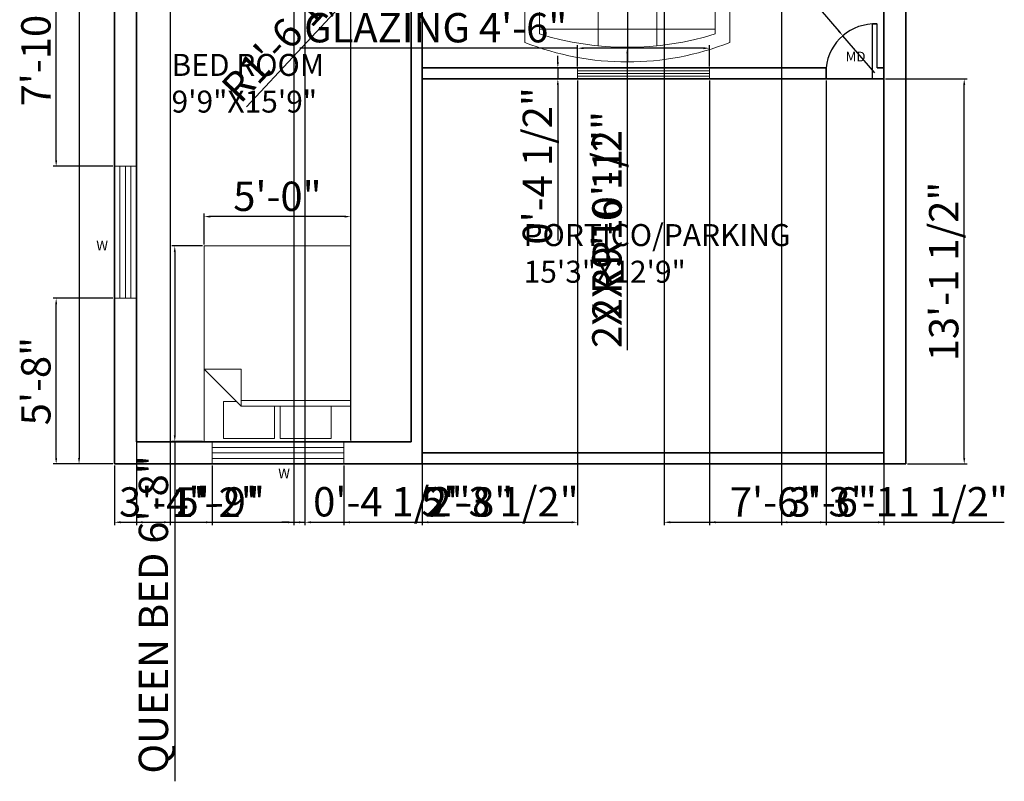
# Model space of a CAD drawing. Units: inches. Extents: x 2691 to 3133, y 1294 to 1993.
# Tile 1 of 7: x 2729 to 3133, y 1294 to 1606. Entities that reach past the tile are written whole.
import ezdxf

# ---------------------------------------------------------------- set-up
doc = ezdxf.new("R2010")
doc.units = ezdxf.units.IN
for name, color, linetype, lineweight in [('A-ANNO-DIMS', 2, 'Continuous', 18), ('A-ANNO-TEXT', 7, 'Continuous', 18), ('A-AREA-IDEN', 7, 'Continuous', 25), ('A-DOOR', 3, 'Continuous', 25), ('A-FURN', 8, 'Continuous', 18), ('A-GLAZ', 4, 'Continuous', 18), ('A-WALL', 7, 'Continuous', 35)]:
    doc.layers.add(name, color=color, linetype=linetype, lineweight=lineweight)
doc.styles.get("Standard").update_dxf_attribs({"font": 'arial.ttf'})
doc.dimstyles.new('ISO-25', dxfattribs={"dimtxt": 12, "dimasz": 2.5, "dimexe": 1.25, "dimexo": 0.625, "dimtad": 1, "dimdec": 1, "dimlunit": 3, "dimtxsty": 'Standard', "dimcen": 2.5, "dimadec": 0, "dimazin": 0, "dimtfac": 1, "dimtdec": 1, "dimtmove": 0, "dimatfit": 3, "dimfxl": 1, "dimarcsym": 0})

# ---------------------------------------------------------------- blocks, each defined once
blk = doc.blocks.new('Window - Wood Frame 36 in. Wide plan')
for p, q in [((0, 6), (0, 0)), ((36, 6), (36, 0)), ((0, 4.5), (36, 4.5)), ((0, 3), (36, 3)), ((0, 1.5), (36, 1.5))]:
    blk.add_line(p, q)
blk = doc.blocks.new('Sofa - Roundback 7 ft.')
for p, q in [((-12.00002, -32.4421), (-12.00003, -6.5971)), ((11.99997, -32.4421), (11.99998, -6.5971)), ((-36.000027, -34), (-36.000027, -11.4696)), ((35.99998, -34), (35.99998, -11.4696)), ((-35.999844, -13.3819), (35.9998, -13.3819)), ((-36.000027, -32.4421), (35.99998, -32.4421))]:
    blk.add_line(p, q)
for points in [[(-36.000027, -34), (-42.000027, -34), (-42.000027, -8)], [(41.99998, -8), (41.99998, -34), (35.99998, -34)]]:
    blk.add_lwpolyline(points)
for centre, radius, start, end in [((0, -114.25), 114.25, 68.43141, 111.5686), ((-0.00001, -127.1968), 121.1968, 72.72033, 107.2797)]:
    blk.add_arc(centre, radius, start, end)
blk = doc.blocks.new('Bed - Queen')
for p, q in [((0, -80.00003), (0, 0)), ((0, 0), (59.99999, 0)), ((59.99999, 0), (59.99999, -80.00003)), ((7.99999, -1.2), (28.79998, -1.2)), ((7.99999, -14.4), (7.99999, -1.2)), ((28.79998, -1.2), (28.79998, -14.4)), ((31.19999, -1.2), (51.99999, -1.2)), ((31.19999, -14.4), (31.19999, -1.2)), ((51.99999, -1.2), (51.99999, -16.4)), ((0, -14.4), (44.8, -14.4)), ((59.99999, -29.6), (44.8, -14.4)), ((44.8, -14.4), (44.8, -29.6)), ((44.8, -16.8), (0, -16.8)), ((51.99999, -16.4), (46.79936, -16.4)), ((44.8, -29.6), (59.99999, -29.6)), ((59.99999, -80.00003), (0, -80.00003))]:
    blk.add_line(p, q)
blk = doc.blocks.new('*D11')
at = {"layer": 'A-ANNO-DIMS', "color": 0, "lineweight": -2, "transparency": 16777216}
for p, q in [((2767.62, 1880.05), (2752.52, 1880.05)), ((2753.77, 1877.55), (2753.77, 1426.55)), ((2767.62, 1424.05), (2752.52, 1424.05))]:
    blk.add_line(p, q, dxfattribs=at)
at = {"layer": 'A-ANNO-DIMS', "color": 0, "transparency": 16777216}
for points in [[(2753.35, 1877.55), (2754.18, 1877.55), (2753.77, 1880.05)], [(2753.35, 1426.55), (2754.18, 1426.55), (2753.77, 1424.05)]]:
    blk.add_solid(points, dxfattribs=at)
at = {"layer": 'Defpoints', "color": 0, "transparency": 16777216}
for p in [(2768.25, 1880.05), (2753.77, 1424.05), (2768.25, 1424.05)]:
    blk.add_point(p, dxfattribs=at)
at = {"layer": 'A-ANNO-DIMS', "color": 0, "transparency": 16777216, "insert": (2747.01, 1652.05), "char_height": 12, "attachment_point": 5, "rotation": 90}
blk.add_mtext("38'", dxfattribs=at)
blk = doc.blocks.new('DOOR-LEAF-WIDE')
for p, q in [((0, 0), (0, 22.5)), ((2, 18), (2, 0)), ((2, 0), (0, 0))]:
    blk.add_line(p, q)
blk = doc.blocks.new('*D16')
at = {"layer": 'A-ANNO-DIMS', "color": 0, "lineweight": -2, "transparency": 16777216}
for p, q in [((2957.85, 1594.15), (2844.15, 1594.15)), ((2957.85, 1586.68), (2957.85, 1595.4)), ((3009.35, 1594.15), (2960.35, 1594.15)), ((3011.85, 1586.68), (3011.85, 1595.4))]:
    blk.add_line(p, q, dxfattribs=at)
at = {"layer": 'A-ANNO-DIMS', "color": 0, "transparency": 16777216}
for points in [[(2960.35, 1594.57), (2960.35, 1593.74), (2957.85, 1594.15)], [(3009.35, 1594.57), (3009.35, 1593.74), (3011.85, 1594.15)]]:
    blk.add_solid(points, dxfattribs=at)
at = {"layer": 'Defpoints', "color": 0, "transparency": 16777216}
for p in [(2957.85, 1594.15), (2957.85, 1586.05), (3011.85, 1586.05)]:
    blk.add_point(p, dxfattribs=at)
at = {"layer": 'A-ANNO-DIMS', "color": 0, "transparency": 16777216, "insert": (2899.75, 1600.98), "char_height": 12, "attachment_point": 5}
blk.add_mtext('GLAZING 4\'-6"', dxfattribs=at)
blk = doc.blocks.new('*D17')
at = {"layer": 'A-ANNO-DIMS', "color": 0, "lineweight": -2, "transparency": 16777216}
for p, q in [((2949.75, 1588.55), (2949.75, 1591.05)), ((2957.22, 1586.05), (2948.5, 1586.05)), ((2949.75, 1586.05), (2949.75, 1581.55)), ((2957.22, 1581.55), (2948.5, 1581.55)), ((2949.75, 1579.05), (2949.75, 1515.44))]:
    blk.add_line(p, q, dxfattribs=at)
at = {"layer": 'A-ANNO-DIMS', "color": 0, "transparency": 16777216}
for points in [[(2949.33, 1588.55), (2950.16, 1588.55), (2949.75, 1586.05)], [(2949.33, 1579.05), (2950.16, 1579.05), (2949.75, 1581.55)]]:
    blk.add_solid(points, dxfattribs=at)
at = {"layer": 'Defpoints', "color": 0, "transparency": 16777216}
for p in [(2957.85, 1586.05), (2949.75, 1581.55), (2957.85, 1581.55)]:
    blk.add_point(p, dxfattribs=at)
at = {"layer": 'A-ANNO-DIMS', "color": 0, "transparency": 16777216, "insert": (2942.92, 1546), "char_height": 12, "attachment_point": 5, "rotation": 90}
blk.add_mtext('0\'-4 1/2"', dxfattribs=at)
blk = doc.blocks.new('*D32')
at = {"layer": 'A-ANNO-DIMS', "color": 0, "lineweight": -2, "transparency": 16777216}
for p, q in [((2804.33, 1513.26), (2791.71, 1513.26)), ((2792.96, 1510.76), (2792.96, 1435.76)), ((2804.33, 1433.26), (2791.71, 1433.26)), ((2792.96, 1433.26), (2792.96, 1294.23))]:
    blk.add_line(p, q, dxfattribs=at)
at = {"layer": 'A-ANNO-DIMS', "color": 0, "transparency": 16777216}
for points in [[(2792.54, 1510.76), (2793.37, 1510.76), (2792.96, 1513.26)], [(2792.54, 1435.76), (2793.37, 1435.76), (2792.96, 1433.26)]]:
    blk.add_solid(points, dxfattribs=at)
at = {"layer": 'Defpoints', "color": 0, "transparency": 16777216}
for p in [(2804.96, 1513.26), (2792.96, 1433.26), (2804.96, 1433.26)]:
    blk.add_point(p, dxfattribs=at)
at = {"layer": 'A-ANNO-DIMS', "color": 0, "transparency": 16777216, "insert": (2785.76, 1362.49), "char_height": 12, "attachment_point": 5, "rotation": 90}
blk.add_mtext('QUEEN BED 6\'-8"', dxfattribs=at)
blk = doc.blocks.new('*D33')
at = {"layer": 'A-ANNO-DIMS', "color": 0, "lineweight": -2, "transparency": 16777216}
for p, q in [((2804.96, 1513.88), (2804.96, 1526.51)), ((2862.46, 1525.26), (2807.46, 1525.26)), ((2864.96, 1513.88), (2864.96, 1526.51))]:
    blk.add_line(p, q, dxfattribs=at)
at = {"layer": 'A-ANNO-DIMS', "color": 0, "transparency": 16777216}
for points in [[(2807.46, 1525.67), (2807.46, 1524.84), (2804.96, 1525.26)], [(2862.46, 1525.67), (2862.46, 1524.84), (2864.96, 1525.26)]]:
    blk.add_solid(points, dxfattribs=at)
at = {"layer": 'Defpoints', "color": 0, "transparency": 16777216}
for p in [(2804.96, 1525.26), (2804.96, 1513.26), (2864.96, 1513.26)]:
    blk.add_point(p, dxfattribs=at)
at = {"layer": 'A-ANNO-DIMS', "color": 0, "transparency": 16777216, "insert": (2834.96, 1532.01), "char_height": 12, "attachment_point": 5}
blk.add_mtext('5\'-0"', dxfattribs=at)
blk = doc.blocks.new('*D41')
at = {"layer": 'A-ANNO-DIMS', "color": 0, "lineweight": -2, "transparency": 16777216}
for p, q in [((2768.25, 1423.43), (2768.25, 1398.95)), ((2808.21, 1423.43), (2808.21, 1398.95)), ((2770.75, 1400.2), (2805.71, 1400.2))]:
    blk.add_line(p, q, dxfattribs=at)
at = {"layer": 'A-ANNO-DIMS', "color": 0, "transparency": 16777216}
for points in [[(2770.75, 1400.62), (2770.75, 1399.79), (2768.25, 1400.2)], [(2805.71, 1400.62), (2805.71, 1399.79), (2808.21, 1400.2)]]:
    blk.add_solid(points, dxfattribs=at)
at = {"layer": 'Defpoints', "color": 0, "transparency": 16777216}
for p in [(2768.25, 1424.05), (2808.21, 1424.05), (2808.21, 1400.2)]:
    blk.add_point(p, dxfattribs=at)
at = {"layer": 'A-ANNO-DIMS', "color": 0, "transparency": 16777216, "insert": (2788.23, 1406.96), "char_height": 12, "attachment_point": 5}
blk.add_mtext('3\'-4"', dxfattribs=at)
blk = doc.blocks.new('*D42')
at = {"layer": 'A-ANNO-DIMS', "color": 0, "lineweight": -2, "transparency": 16777216}
for p, q in [((2862.21, 1423.43), (2862.21, 1398.95)), ((2894.25, 1423.43), (2894.25, 1398.95)), ((2864.71, 1400.2), (2891.75, 1400.2)), ((2894.25, 1400.2), (2930.1, 1400.2))]:
    blk.add_line(p, q, dxfattribs=at)
at = {"layer": 'A-ANNO-DIMS', "color": 0, "transparency": 16777216}
for points in [[(2864.71, 1400.62), (2864.71, 1399.79), (2862.21, 1400.2)], [(2891.75, 1400.62), (2891.75, 1399.79), (2894.25, 1400.2)]]:
    blk.add_solid(points, dxfattribs=at)
at = {"layer": 'Defpoints', "color": 0, "transparency": 16777216}
for p in [(2862.21, 1424.05), (2894.25, 1424.05), (2894.25, 1400.2)]:
    blk.add_point(p, dxfattribs=at)
at = {"layer": 'A-ANNO-DIMS', "color": 0, "transparency": 16777216, "insert": (2913.43, 1406.96), "char_height": 12, "attachment_point": 5}
blk.add_mtext('2\'-8"', dxfattribs=at)
blk = doc.blocks.new('*D43')
at = {"layer": 'A-ANNO-DIMS', "color": 0, "lineweight": -2, "transparency": 16777216}
for p, q in [((2767.62, 1491.83), (2743.15, 1491.83)), ((2744.4, 1426.55), (2744.4, 1489.33)), ((2767.62, 1424.05), (2743.15, 1424.05))]:
    blk.add_line(p, q, dxfattribs=at)
at = {"layer": 'A-ANNO-DIMS', "color": 0, "transparency": 16777216}
for points in [[(2743.98, 1489.33), (2744.82, 1489.33), (2744.4, 1491.83)], [(2743.98, 1426.55), (2744.82, 1426.55), (2744.4, 1424.05)]]:
    blk.add_solid(points, dxfattribs=at)
at = {"layer": 'Defpoints', "color": 0, "transparency": 16777216}
for p in [(2744.4, 1491.83), (2768.25, 1491.83), (2768.25, 1424.05)]:
    blk.add_point(p, dxfattribs=at)
at = {"layer": 'A-ANNO-DIMS', "color": 0, "transparency": 16777216, "insert": (2737.65, 1457.94), "char_height": 12, "attachment_point": 5, "rotation": 90}
blk.add_mtext('5\'-8"', dxfattribs=at)
blk = doc.blocks.new('*D44')
at = {"layer": 'A-ANNO-DIMS', "color": 0, "lineweight": -2, "transparency": 16777216}
for p, q in [((2776.62, 1640.05), (2743.15, 1640.05)), ((2744.4, 1548.33), (2744.4, 1637.55)), ((2767.62, 1545.83), (2743.15, 1545.83))]:
    blk.add_line(p, q, dxfattribs=at)
at = {"layer": 'A-ANNO-DIMS', "color": 0, "transparency": 16777216}
for points in [[(2743.98, 1637.55), (2744.82, 1637.55), (2744.4, 1640.05)], [(2743.98, 1548.33), (2744.82, 1548.33), (2744.4, 1545.83)]]:
    blk.add_solid(points, dxfattribs=at)
at = {"layer": 'Defpoints', "color": 0, "transparency": 16777216}
for p in [(2744.4, 1640.05), (2777.25, 1640.05), (2768.25, 1545.83)]:
    blk.add_point(p, dxfattribs=at)
at = {"layer": 'A-ANNO-DIMS', "color": 0, "transparency": 16777216, "insert": (2737.65, 1592.94), "char_height": 12, "attachment_point": 5, "rotation": 90}
blk.add_mtext('7\'-10"', dxfattribs=at)
blk = doc.blocks.new('*D47')
at = {"layer": 'A-ANNO-DIMS', "color": 0, "lineweight": -2, "transparency": 16777216}
for p, q in [((3083.87, 1581.55), (3117.35, 1581.55)), ((3116.1, 1426.55), (3116.1, 1579.05)), ((3092.87, 1424.05), (3117.35, 1424.05))]:
    blk.add_line(p, q, dxfattribs=at)
at = {"layer": 'A-ANNO-DIMS', "color": 0, "transparency": 16777216}
for points in [[(3115.68, 1579.05), (3116.52, 1579.05), (3116.1, 1581.55)], [(3115.68, 1426.55), (3116.52, 1426.55), (3116.1, 1424.05)]]:
    blk.add_solid(points, dxfattribs=at)
at = {"layer": 'Defpoints', "color": 0, "transparency": 16777216}
for p in [(3083.25, 1581.55), (3116.1, 1581.55), (3092.25, 1424.05)]:
    blk.add_point(p, dxfattribs=at)
at = {"layer": 'A-ANNO-DIMS', "color": 0, "transparency": 16777216, "insert": (3109.27, 1502.8), "char_height": 12, "attachment_point": 5, "rotation": 90}
blk.add_mtext('13\'-1 1/2"', dxfattribs=at)
blk = doc.blocks.new('*D48')
at = {"layer": 'A-ANNO-DIMS', "color": 0, "lineweight": -2, "transparency": 16777216}
for p, q in [((2894.25, 1580.93), (2894.25, 1398.95)), ((2957.85, 1580.93), (2957.85, 1398.95)), ((2896.75, 1400.2), (2955.35, 1400.2))]:
    blk.add_line(p, q, dxfattribs=at)
at = {"layer": 'A-ANNO-DIMS', "color": 0, "transparency": 16777216}
for points in [[(2896.75, 1400.62), (2896.75, 1399.79), (2894.25, 1400.2)], [(2955.35, 1400.62), (2955.35, 1399.79), (2957.85, 1400.2)]]:
    blk.add_solid(points, dxfattribs=at)
at = {"layer": 'Defpoints', "color": 0, "transparency": 16777216}
for p in [(2894.25, 1581.55), (2957.85, 1581.55), (2957.85, 1400.2)]:
    blk.add_point(p, dxfattribs=at)
at = {"layer": 'A-ANNO-DIMS', "color": 0, "transparency": 16777216, "insert": (2926.05, 1407.04), "char_height": 12, "attachment_point": 5}
blk.add_mtext('5\'-3 1/2"', dxfattribs=at)
blk = doc.blocks.new('*D49')
at = {"layer": 'A-ANNO-DIMS', "color": 0, "lineweight": -2, "transparency": 16777216}
for p, q in [((2993.25, 1870.43), (2993.25, 1398.95)), ((3083.25, 1870.43), (3083.25, 1398.95)), ((2995.75, 1400.2), (3080.75, 1400.2))]:
    blk.add_line(p, q, dxfattribs=at)
at = {"layer": 'A-ANNO-DIMS', "color": 0, "transparency": 16777216}
for points in [[(2995.75, 1400.62), (2995.75, 1399.79), (2993.25, 1400.2)], [(3080.75, 1400.62), (3080.75, 1399.79), (3083.25, 1400.2)]]:
    blk.add_solid(points, dxfattribs=at)
at = {"layer": 'Defpoints', "color": 0, "transparency": 16777216}
for p in [(2993.25, 1871.05), (3083.25, 1871.05), (3083.25, 1400.2)]:
    blk.add_point(p, dxfattribs=at)
at = {"layer": 'A-ANNO-DIMS', "color": 0, "transparency": 16777216, "insert": (3038.25, 1406.96), "char_height": 12, "attachment_point": 5}
blk.add_mtext('7\'-6"', dxfattribs=at)
blk = doc.blocks.new('*D52')
at = {"layer": 'A-ANNO-DIMS', "color": 0, "lineweight": -2, "transparency": 16777216}
for p, q in [((3041.25, 1747.43), (3041.25, 1398.95)), ((3083.25, 1747.43), (3083.25, 1398.95)), ((3043.75, 1400.2), (3080.75, 1400.2))]:
    blk.add_line(p, q, dxfattribs=at)
at = {"layer": 'A-ANNO-DIMS', "color": 0, "transparency": 16777216}
for points in [[(3043.75, 1400.62), (3043.75, 1399.79), (3041.25, 1400.2)], [(3080.75, 1400.62), (3080.75, 1399.79), (3083.25, 1400.2)]]:
    blk.add_solid(points, dxfattribs=at)
at = {"layer": 'Defpoints', "color": 0, "transparency": 16777216}
for p in [(3041.25, 1748.05), (3083.25, 1748.05), (3083.25, 1400.2)]:
    blk.add_point(p, dxfattribs=at)
at = {"layer": 'A-ANNO-DIMS', "color": 0, "transparency": 16777216, "insert": (3062.25, 1406.96), "char_height": 12, "attachment_point": 5}
blk.add_mtext('3\'-6"', dxfattribs=at)
blk = doc.blocks.new('*D53')
at = {"layer": 'A-ANNO-DIMS', "color": 0, "lineweight": -2, "transparency": 16777216}
for p, q in [((3011.85, 1580.93), (3011.85, 1398.95)), ((3059.53, 1580.93), (3059.53, 1398.95)), ((3014.35, 1400.2), (3057.03, 1400.2)), ((3059.53, 1400.2), (3132.46, 1400.2))]:
    blk.add_line(p, q, dxfattribs=at)
at = {"layer": 'A-ANNO-DIMS', "color": 0, "transparency": 16777216}
for points in [[(3014.35, 1400.62), (3014.35, 1399.79), (3011.85, 1400.2)], [(3057.03, 1400.62), (3057.03, 1399.79), (3059.53, 1400.2)]]:
    blk.add_solid(points, dxfattribs=at)
at = {"layer": 'Defpoints', "color": 0, "transparency": 16777216}
for p in [(3011.85, 1581.55), (3059.53, 1581.55), (3059.53, 1400.2)]:
    blk.add_point(p, dxfattribs=at)
at = {"layer": 'A-ANNO-DIMS', "color": 0, "transparency": 16777216, "insert": (3097.25, 1407.04), "char_height": 12, "attachment_point": 5}
blk.add_mtext('3\'-11 1/2"', dxfattribs=at)
blk = doc.blocks.new('*D55')
at = {"layer": 'A-ANNO-DIMS', "color": 0, "lineweight": -2, "transparency": 16777216}
for p, q in [((2841.75, 1643.93), (2841.75, 1398.95)), ((2846.25, 1643.93), (2846.25, 1398.95)), ((2839.25, 1400.2), (2836.75, 1400.2)), ((2841.75, 1400.2), (2846.25, 1400.2)), ((2848.75, 1400.2), (2912.36, 1400.2))]:
    blk.add_line(p, q, dxfattribs=at)
at = {"layer": 'A-ANNO-DIMS', "color": 0, "transparency": 16777216}
for points in [[(2839.25, 1400.62), (2839.25, 1399.79), (2841.75, 1400.2)], [(2848.75, 1400.62), (2848.75, 1399.79), (2846.25, 1400.2)]]:
    blk.add_solid(points, dxfattribs=at)
at = {"layer": 'Defpoints', "color": 0, "transparency": 16777216}
for p in [(2841.75, 1644.55), (2846.25, 1644.55), (2846.25, 1400.2)]:
    blk.add_point(p, dxfattribs=at)
at = {"layer": 'A-ANNO-DIMS', "color": 0, "transparency": 16777216, "insert": (2881.8, 1407.03), "char_height": 12, "attachment_point": 5}
blk.add_mtext('0\'-4 1/2"', dxfattribs=at)
blk = doc.blocks.new('*D56')
at = {"layer": 'A-ANNO-DIMS', "color": 0, "lineweight": -2, "transparency": 16777216}
for p, q in [((2846.25, 1643.93), (2846.25, 1398.95)), ((2777.25, 1639.43), (2777.25, 1398.95)), ((2779.75, 1400.2), (2843.75, 1400.2))]:
    blk.add_line(p, q, dxfattribs=at)
at = {"layer": 'A-ANNO-DIMS', "color": 0, "transparency": 16777216}
for points in [[(2779.75, 1400.62), (2779.75, 1399.79), (2777.25, 1400.2)], [(2843.75, 1400.62), (2843.75, 1399.79), (2846.25, 1400.2)]]:
    blk.add_solid(points, dxfattribs=at)
at = {"layer": 'Defpoints', "color": 0, "transparency": 16777216}
for p in [(2846.25, 1644.55), (2777.25, 1640.05), (2846.25, 1400.2)]:
    blk.add_point(p, dxfattribs=at)
at = {"layer": 'A-ANNO-DIMS', "color": 0, "transparency": 16777216, "insert": (2811.75, 1406.96), "char_height": 12, "attachment_point": 5}
blk.add_mtext('5\'-9"', dxfattribs=at)
blk = doc.blocks.new('*D58')
at = {"layer": 'A-ANNO-DIMS', "color": 0, "lineweight": -2, "transparency": 16777216}
for p, q in [((2777.25, 1756.43), (2777.25, 1398.95)), ((2791.1, 1756.43), (2791.1, 1398.95)), ((2779.75, 1400.2), (2788.6, 1400.2)), ((2791.1, 1400.2), (2825.62, 1400.2))]:
    blk.add_line(p, q, dxfattribs=at)
at = {"layer": 'A-ANNO-DIMS', "color": 0, "transparency": 16777216}
for points in [[(2779.75, 1400.62), (2779.75, 1399.79), (2777.25, 1400.2)], [(2788.6, 1400.62), (2788.6, 1399.79), (2791.1, 1400.2)]]:
    blk.add_solid(points, dxfattribs=at)
at = {"layer": 'Defpoints', "color": 0, "transparency": 16777216}
for p in [(2777.25, 1757.05), (2791.1, 1757.05), (2791.1, 1400.2)]:
    blk.add_point(p, dxfattribs=at)
at = {"layer": 'A-ANNO-DIMS', "color": 0, "transparency": 16777216, "insert": (2809.61, 1406.85), "char_height": 12, "attachment_point": 5}
blk.add_mtext('1\'-2"', dxfattribs=at)
blk = doc.blocks.new('*D61')
at = {"layer": 'A-ANNO-DIMS', "color": 0, "lineweight": -2, "transparency": 16777216}
for p, q in [((2864.96, 1433.88), (2864.96, 1905.15)), ((2867.46, 1903.9), (2887.25, 1903.9)), ((2889.75, 1433.68), (2889.75, 1905.15)), ((2889.75, 1903.9), (2925.6, 1903.9))]:
    blk.add_line(p, q, dxfattribs=at)
at = {"layer": 'A-ANNO-DIMS', "color": 0, "transparency": 16777216}
for points in [[(2867.46, 1904.32), (2867.46, 1903.49), (2864.96, 1903.9)], [(2887.25, 1904.32), (2887.25, 1903.49), (2889.75, 1903.9)]]:
    blk.add_solid(points, dxfattribs=at)
at = {"layer": 'Defpoints', "color": 0, "transparency": 16777216}
for p in [(2889.75, 1903.9), (2864.96, 1433.26), (2889.75, 1433.05)]:
    blk.add_point(p, dxfattribs=at)
at = {"layer": 'A-ANNO-DIMS', "color": 0, "transparency": 16777216, "insert": (2908.93, 1910.55), "char_height": 12, "attachment_point": 5}
blk.add_mtext('2\'-1"', dxfattribs=at)
blk = doc.blocks.new('*D62')
at = {"layer": 'A-ANNO-DIMS', "color": 0, "lineweight": -2, "transparency": 16777216}
for p, q in [((3034.07, 1636.88), (3064.78, 1601.13)), ((3079.48, 1584.03), (3066.41, 1599.24))]:
    blk.add_line(p, q, dxfattribs=at)
at = {"layer": 'A-ANNO-DIMS', "color": 0, "transparency": 16777216}
blk.add_solid([(3065.1, 1601.4), (3064.47, 1600.86), (3066.41, 1599.24)], dxfattribs=at)
at = {"layer": 'Defpoints', "color": 0, "transparency": 16777216}
for p in [(3066.41, 1599.24), (3079.48, 1584.03)]:
    blk.add_point(p, dxfattribs=at)
at = {"layer": 'A-ANNO-DIMS', "color": 0, "transparency": 16777216, "insert": (3053.73, 1624.36), "char_height": 12, "attachment_point": 5, "rotation": 310.6735}
blk.add_mtext('R1\'-8"', dxfattribs=at)
blk = doc.blocks.new('*D63')
at = {"layer": 'A-ANNO-DIMS', "color": 0, "lineweight": -2, "transparency": 16777216}
for p, q in [((2887.75, 1640.32), (2875.27, 1626.95)), ((2822.33, 1570.22), (2873.57, 1625.12))]:
    blk.add_line(p, q, dxfattribs=at)
at = {"layer": 'A-ANNO-DIMS', "color": 0, "transparency": 16777216}
blk.add_solid([(2873.26, 1625.4), (2873.87, 1624.83), (2875.27, 1626.95)], dxfattribs=at)
at = {"layer": 'Defpoints', "color": 0, "transparency": 16777216}
for p in [(2887.75, 1640.32), (2875.27, 1626.95)]:
    blk.add_point(p, dxfattribs=at)
at = {"layer": 'A-ANNO-DIMS', "color": 0, "transparency": 16777216, "insert": (2842.1, 1601.41), "char_height": 12, "attachment_point": 5, "rotation": 46.9754}
blk.add_mtext('R1\'-6 1/2"', dxfattribs=at)
blk = doc.blocks.new('*D66')
at = {"layer": 'A-ANNO-DIMS', "color": 0, "lineweight": -2, "transparency": 16777216}
for p, q in [((2978.21, 1715.72), (2978.21, 1594.52)), ((2978.21, 1481.83), (2978.21, 1592.02))]:
    blk.add_line(p, q, dxfattribs=at)
at = {"layer": 'A-ANNO-DIMS', "color": 0, "transparency": 16777216}
blk.add_solid([(2977.79, 1592.02), (2978.62, 1592.02), (2978.21, 1594.52)], dxfattribs=at)
at = {"layer": 'Defpoints', "color": 0, "transparency": 16777216}
for p in [(2978.21, 1715.72), (2978.21, 1594.52)]:
    blk.add_point(p, dxfattribs=at)
at = {"layer": 'A-ANNO-DIMS', "color": 0, "transparency": 16777216, "insert": (2971.46, 1521.8), "char_height": 12, "attachment_point": 5, "rotation": 89.9999}
blk.add_mtext('2X R10\'-1"', dxfattribs=at)
blk = doc.blocks.new('*D67')
at = {"layer": 'A-ANNO-DIMS', "color": 0, "lineweight": -2, "transparency": 16777216}
for p, q in [((2978.21, 1702.77), (2978.21, 1588.52)), ((2978.21, 1470.68), (2978.21, 1586.02))]:
    blk.add_line(p, q, dxfattribs=at)
at = {"layer": 'A-ANNO-DIMS', "color": 0, "transparency": 16777216}
blk.add_solid([(2977.79, 1586.02), (2978.62, 1586.02), (2978.21, 1588.52)], dxfattribs=at)
at = {"layer": 'Defpoints', "color": 0, "transparency": 16777216}
for p in [(2978.21, 1702.77), (2978.21, 1588.52)]:
    blk.add_point(p, dxfattribs=at)
at = {"layer": 'A-ANNO-DIMS', "color": 0, "transparency": 16777216, "insert": (2971.38, 1519.97), "char_height": 12, "attachment_point": 5, "rotation": 89.9999}
blk.add_mtext('2X R9\'-6 1/2"', dxfattribs=at)

msp = doc.modelspace()

# ---------------------------------------------------------------- linework, layer by layer
at = {"layer": 'A-DOOR'}
msp.add_arc((3079.48, 1584.03), 20.05, 87.1409, 174.2088, dxfattribs=at)
at = {"layer": 'A-WALL'}
for p, q in [((2768.25, 1880.05), (2768.25, 1424.05)), ((3092.25, 1424.05), (3092.25, 1880.05)), ((3083.25, 1433.05), (3083.25, 1871.05)), ((2889.75, 1644.55), (2889.75, 1433.05)), ((2894.25, 1644.55), (2894.25, 1424.05)), ((2777.25, 1640.05), (2777.25, 1433.05)), ((2894.25, 1586.05), (3059.53, 1586.05)), ((3059.53, 1586.05), (3059.53, 1581.55)), ((3080.48, 1586.05), (3083.25, 1586.05)), ((2894.25, 1581.55), (3083.25, 1581.55)), ((3078.48, 1581.55), (3061.11, 1581.55)), ((2777.25, 1433.05), (2889.75, 1433.05)), ((3083.25, 1433.05), (3083.25, 1424.05)), ((3083.25, 1428.55), (2894.25, 1428.55)), ((3083.25, 1424.05), (3083.25, 1428.55)), ((2768.25, 1424.05), (2894.25, 1424.05)), ((2894.25, 1424.05), (3083.25, 1424.05)), ((3083.25, 1424.05), (3092.25, 1424.05))]:
    msp.add_line(p, q, dxfattribs=at)

# ---------------------------------------------------------------- block references
at = {"layer": 'A-DOOR', "extrusion": (0, 0, -1), "zscale": -1, "rotation": 180}
msp.add_blockref('DOOR-LEAF-WIDE', (-3078.48, 1604.05), dxfattribs=at)
at = {"layer": 'A-FURN', "rotation": 180}
for name, p in [('Sofa - Roundback 7 ft.', (2978.21, 1588.52)), ('Bed - Queen', (2864.96, 1433.26))]:
    msp.add_blockref(name, p, dxfattribs=at)
at = {"layer": 'A-GLAZ', "xscale": 1.5}
for p, yscale, rotation in [((3011.85, 1586.05), 0.75, 180), ((2777.25, 1491.83), 1.5, 90)]:
    msp.add_blockref('Window - Wood Frame 36 in. Wide plan', p, dxfattribs=dict(at, yscale=yscale, rotation=rotation))
at = {"layer": 'A-GLAZ', "xscale": 1.5, "yscale": 1.5}
msp.add_blockref('Window - Wood Frame 36 in. Wide plan', (2808.21, 1424.05), dxfattribs=at)

# ---------------------------------------------------------------- texts
at = {"layer": 'A-ANNO-TEXT', "char_height": 4, "attachment_point": 1}
for s, insert in [('MD', (3067.52, 1592.72)), ('W', (2760.83, 1515.39)), ('W', (2835.3, 1422.18))]:
    msp.add_mtext_dynamic_manual_height_columns(s, width=0.1038, gutter_width=12.5, heights=[0], dxfattribs=dict(at, insert=insert))
at = {"layer": 'A-AREA-IDEN', "insert": (2791.62, 1591.81), "char_height": 9, "attachment_point": 1}
msp.add_mtext('BED ROOM \\P9\'9"X15\'9"', dxfattribs=at)
at = {"layer": 'A-AREA-IDEN', "insert": (2935.74, 1522.2), "char_height": 9, "width": 257.4045, "attachment_point": 1}
msp.add_mtext('PORTICO/PARKING\\P15\'3"X12\'9"', dxfattribs=at)

# ---------------------------------------------------------------- dimensions: what is measured, and where the dimension line sits
at = {"layer": 'A-ANNO-DIMS'}
for base, p1, p2, picture, middle in [((2889.75, 1903.9), (2864.96, 1433.26), (2889.75, 1433.05), '*D61', (2908.93, 1910.55)), ((3083.25, 1400.2), (2993.25, 1871.05), (3083.25, 1871.05), '*D49', (3038.25, 1406.96)), ((2791.0965, 1400.2049), (2777.2496, 1757.0549), (2791.0965, 1757.0549), '*D58', (2809.6063, 1406.8545)), ((3083.25, 1400.2), (3041.25, 1748.05), (3083.25, 1748.05), '*D52', (3062.25, 1406.96)), ((2846.25, 1400.2), (2777.25, 1640.05), (2846.25, 1644.55), '*D56', (2811.75, 1406.96)), ((2846.25, 1400.2), (2841.75, 1644.55), (2846.25, 1644.55), '*D55', (2881.8, 1407.03)), ((2957.85, 1400.2), (2894.25, 1581.55), (2957.85, 1581.55), '*D48', (2926.05, 1407.04)), ((3059.53, 1400.2), (3011.85, 1581.55), (3059.53, 1581.55), '*D53', (3097.25, 1407.04)), ((2808.21, 1400.2), (2768.25, 1424.05), (2808.21, 1424.05), '*D41', (2788.23, 1406.96)), ((2894.25, 1400.2), (2862.21, 1424.05), (2894.25, 1424.05), '*D42', (2913.43, 1406.96))]:
    dim = msp.add_linear_dim(base=base, p1=p1, p2=p2, dimstyle='ISO-25', override={"dimdec": 1, "dimlfac": 1, "dimrnd": 0, "dimzin": 1, "dimdsep": 46, "dimlunit": 4, "dimfrac": 2}, dxfattribs=at)
    dim.commit()
    dim.dimension.update_dxf_attribs({"geometry": picture, "text_midpoint": middle})
for base, p1, p2, angle, override, picture, middle in [((2753.77, 1424.05), (2768.25, 1880.05), (2768.25, 1424.05), 90, {"dimclrd": 0, "dimclre": 0, "dimclrt": 0}, '*D11', (2747.01, 1652.05)), ((2744.4, 1640.05), (2768.25, 1545.83), (2777.25, 1640.05), 90, {"dimdec": 1, "dimlfac": 1, "dimrnd": 0, "dimzin": 1, "dimdsep": 46, "dimlunit": 4, "dimfrac": 2}, '*D44', (2737.65, 1592.94)), ((2949.75, 1581.55), (2957.85, 1586.05), (2957.85, 1581.55), 270, {"dimdec": 1, "dimlfac": 1, "dimrnd": 0, "dimzin": 1, "dimdsep": 46, "dimlunit": 4, "dimfrac": 2}, '*D17', (2942.92, 1546)), ((3116.1, 1581.55), (3092.25, 1424.05), (3083.25, 1581.55), 90, {"dimdec": 1, "dimlfac": 1, "dimrnd": 0, "dimzin": 1, "dimdsep": 46, "dimlunit": 4, "dimfrac": 2}, '*D47', (3109.27, 1502.8)), ((2804.96, 1525.26), (2864.96, 1513.26), (2804.96, 1513.26), 180, {"dimdec": 1, "dimlfac": 1, "dimrnd": 0, "dimzin": 1, "dimdsep": 46, "dimlunit": 4, "dimfrac": 2}, '*D33', (2834.96, 1532.01)), ((2744.4, 1491.83), (2768.25, 1424.05), (2768.25, 1491.83), 90, {"dimdec": 1, "dimlfac": 1, "dimrnd": 0, "dimzin": 1, "dimdsep": 46, "dimlunit": 4, "dimfrac": 2}, '*D43', (2737.65, 1457.94))]:
    dim = msp.add_linear_dim(base=base, p1=p1, p2=p2, angle=angle, dimstyle='ISO-25', override=override, dxfattribs=at)
    dim.commit()
    dim.dimension.update_dxf_attribs({"geometry": picture, "text_midpoint": middle})
for center, mpoint, picture, middle in [((2978.21, 1715.72), (2978.21, 1594.52), '*D66', (2978.21, 1521.8)), ((2978.207141, 1702.768761), (2978.207, 1588.518761), '*D67', (2978.2069154, 1519.968761))]:
    dim = msp.add_radius_dim(center=center, mpoint=mpoint, text='2X <>', dimstyle='ISO-25', override={"dimdec": 1, "dimlfac": 1, "dimrnd": 0, "dimzin": 1, "dimdsep": 46, "dimlunit": 4, "dimfrac": 2}, dxfattribs=at)
    dim.commit()
    dim.dimension.update_dxf_attribs({"geometry": picture, "text_midpoint": middle, "dimtype": 164})
for center, mpoint, picture, middle in [((3079.4801, 1584.0321), (3066.4139, 1599.2371), '*D62', (3053.7312, 1624.3556)), ((2887.75, 1640.32), (2875.27, 1626.95), '*D63', (2842.1, 1601.41))]:
    dim = msp.add_radius_dim(center=center, mpoint=mpoint, dimstyle='ISO-25', override={"dimdec": 1, "dimlfac": 1, "dimrnd": 0, "dimzin": 1, "dimdsep": 46, "dimlunit": 4, "dimfrac": 2}, dxfattribs=at)
    dim.commit()
    dim.dimension.update_dxf_attribs({"geometry": picture, "text_midpoint": middle})
for base, p1, p2, angle, text, picture, middle in [((2957.85, 1594.15), (3011.85, 1586.05), (2957.85, 1586.05), 180, 'GLAZING <>', '*D16', (2899.75, 1600.98)), ((2792.96, 1433.26), (2804.96, 1513.26), (2804.96, 1433.26), 270, 'QUEEN BED <>', '*D32', (2785.76, 1362.49))]:
    dim = msp.add_linear_dim(base=base, p1=p1, p2=p2, angle=angle, text=text, dimstyle='ISO-25', override={"dimdec": 1, "dimlfac": 1, "dimrnd": 0, "dimzin": 1, "dimdsep": 46, "dimlunit": 4, "dimfrac": 2}, dxfattribs=at)
    dim.commit()
    dim.dimension.update_dxf_attribs({"geometry": picture, "text_midpoint": middle})

doc.saveas('drawing.dxf')
